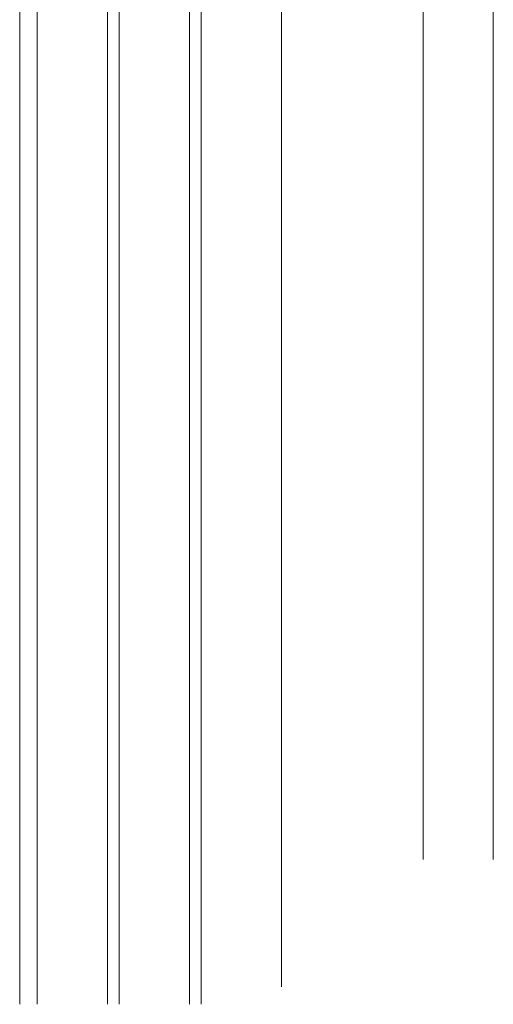
# Model space of a CAD drawing. Units: inches. Extents: x 2443635 to 2446153, y 1826255 to 1827341.
# Tile 11 of 16: x 2445263 to 2445506, y 1826255 to 1826759. Entities that reach past the tile are written whole.
import ezdxf

# ---------------------------------------------------------------- set-up
doc = ezdxf.new("R2010")
doc.units = ezdxf.units.IN
doc.layers.add('A-REFR', color=8, linetype='Continuous', lineweight=13)

msp = doc.modelspace()

# ---------------------------------------------------------------- linework, layer by layer
at = {"layer": 'A-REFR'}
for p, q in [((2445469.966, 1827104.133), (2445469.966, 1826329.288)), ((2445505.966, 1827104.133), (2445505.966, 1826329.288)), ((2445272.466, 1827039.133), (2445272.466, 1826255.288)), ((2445314.466, 1827039.133), (2445314.466, 1826255.288)), ((2445397.466, 1827039.133), (2445397.466, 1826264.288)), ((2445263.466, 1827030.133), (2445263.466, 1826255.288)), ((2445308.466, 1827030.133), (2445308.466, 1826255.288)), ((2445350.466, 1827030.133), (2445350.466, 1826255.288)), ((2445356.466, 1827030.133), (2445356.466, 1826255.288))]:
    msp.add_line(p, q, dxfattribs=at)
at = {"layer": 'A-REFR', "transparency": 33554687}
for p in [(2445227.466, 1827321.207), (2445222.466, 1827316.303)]:
    msp.add_ray(p, (0, -1), dxfattribs=at)

doc.saveas('drawing.dxf')
